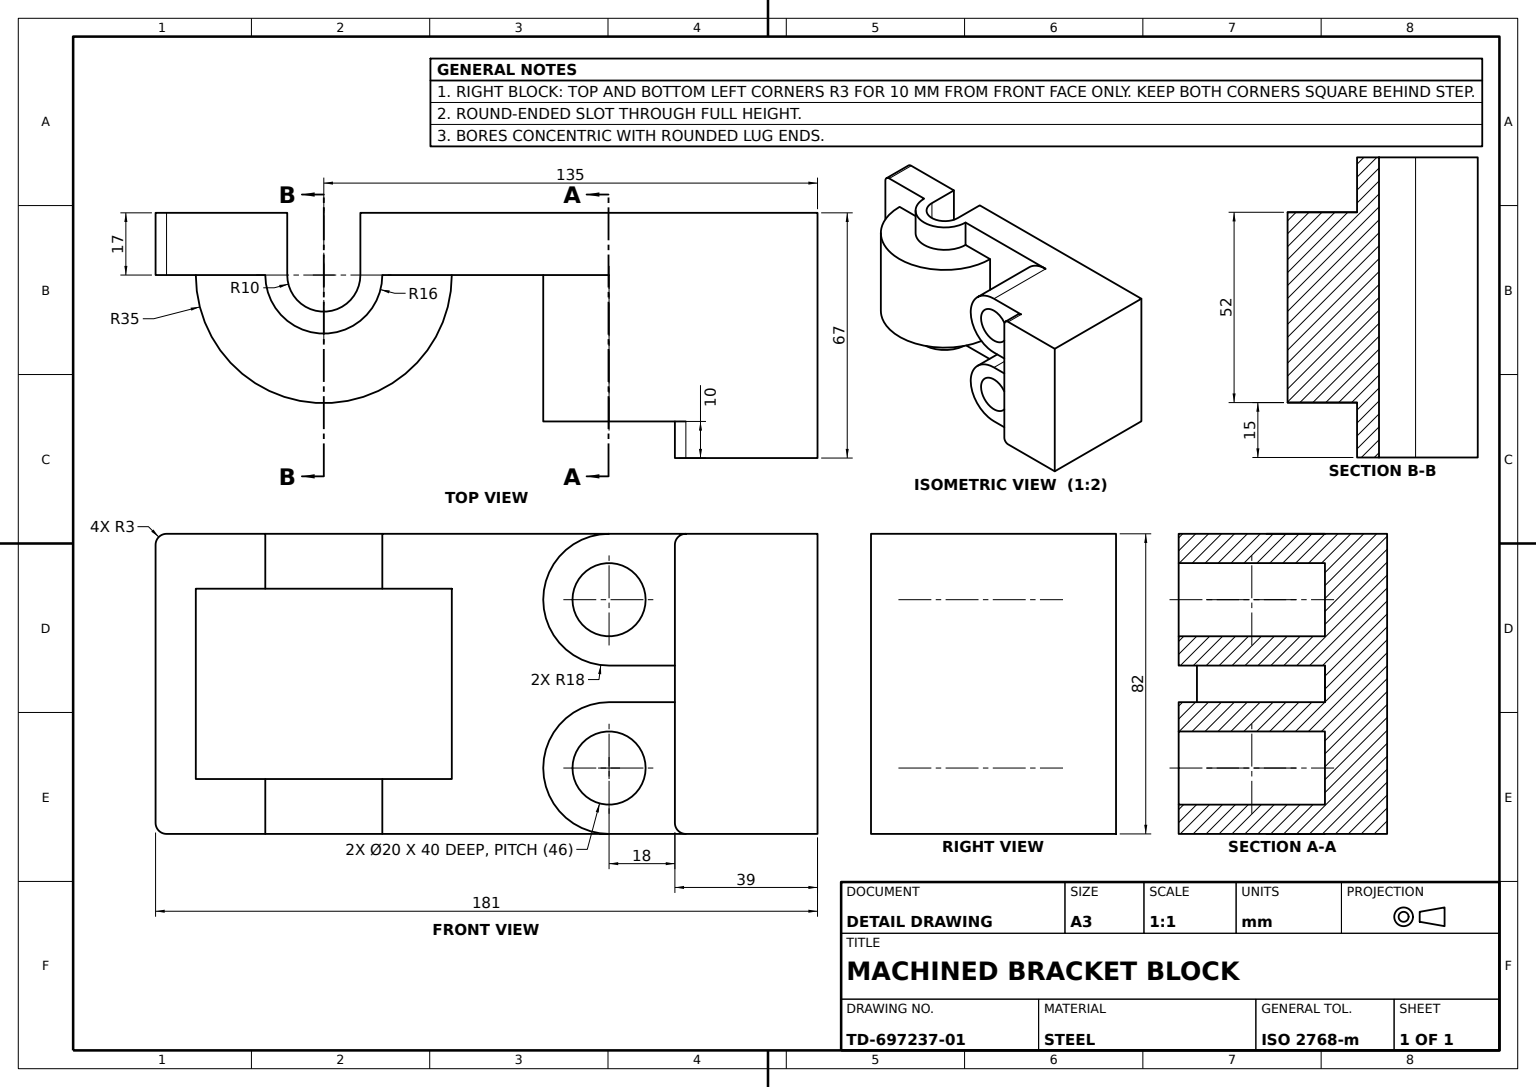
from build123d import *

# Parameters (mm, degrees)
BASE_BLOCK_SKETCH_W       = 175
BASE_BLOCK_SKETCH_H       = 82
BASE_BLOCK_DEPTH          = 17
SIDE_WALL_DEPTH           = 50
STEP_PAD_SKETCH_W         = 17
STEP_PAD_SKETCH_H         = 82
STEP_PAD_DEPTH            = 3
RAISED_BLOCK_DEPTH        = 17
LUG_BOSS_DEPTH            = 82
LUG_PROFILE_CUT_DEPTH     = 82
KNUCKLE_SLOT_1_DEPTH      = 15
KNUCKLE_START             = -15
KNUCKLE_SLOT_2_DEPTH      = 15
KNUCKLE_RING_2_DEPTH      = 15
KNUCKLE_START_2           = 15
KNUCKLE_RING_1_DEPTH      = 15
CURVED_BRACKET_DEPTH      = 40
BRACKET_TRIM_CUT_SKETCH_R = 10
BRACKET_TRIM_CUT_DEPTH    = 40


with BuildPart() as part:
    # Base Block Sketch → Base Block (new body)
    with BuildSketch(Plane.XY):
        with Locations((87.5, 41)):
            Rectangle(BASE_BLOCK_SKETCH_W, BASE_BLOCK_SKETCH_H)
    extrude(amount=BASE_BLOCK_DEPTH)

    # Side Wall Sketch → Side Wall (add)
    with BuildSketch(Plane.XY.offset(17)):
        with BuildLine():
            Line((175, 82), (175, 0))
            Line((175, 0), (139, 0))
            ThreePointArc((139, 0), (136.878679656, 0.878679656), (136, 3))
            Line((136, 3), (136, 79))
            ThreePointArc((136, 79), (136.878679656, 81.121320344), (139, 82))
            Line((139, 82), (175, 82))
        make_face()
    extrude(amount=SIDE_WALL_DEPTH)

    # Step Pad Sketch → Step Pad (add)
    with BuildSketch(Plane.ZY):
        with Locations((8.5, 41)):
            Rectangle(STEP_PAD_SKETCH_W, STEP_PAD_SKETCH_H)
    extrude(amount=STEP_PAD_DEPTH)

    # Raised Block Sketch → Raised Block (add)
    with BuildSketch(Plane.XY.offset(17)):
        with BuildLine():
            Line((-3, 82), (-3, 0))
            ThreePointArc((-3, 0), (-5.121320344, 0.878679656), (-6, 3))
            Line((-6, 3), (-6, 79))
            ThreePointArc((-6, 79), (-5.121320344, 81.121320344), (-3, 82))
        make_face()
    extrude(amount=-RAISED_BLOCK_DEPTH)

    # Lug Boss Sketch → Lug Boss (add)
    with BuildSketch(Plane.XZ):
        with BuildLine():
            ThreePointArc((75, 17), (40, 52), (5, 17))
            Line((5, 17), (75, 17))
        make_face()
    extrude(amount=-LUG_BOSS_DEPTH)

    # Lug Profile Cut Sketch → Lug Profile Cut (cut)
    with BuildSketch(Plane.XZ):
        with BuildLine():
            Line((30, 0), (50, 0))
            Line((50, 0), (50, 17))
            ThreePointArc((50, 17), (40, 27), (30, 17))
            Line((30, 17), (30, 0))
        make_face()
    extrude(amount=-LUG_PROFILE_CUT_DEPTH, mode=Mode.SUBTRACT)

    # Knuckle Slot 1 Sketch → Knuckle Slot 1 (cut)
    with BuildSketch(Plane.XZ):
        with BuildLine():
            Line((5, 17), (30, 17))
            ThreePointArc((30, 17), (40, 27), (50, 17))
            Line((50, 17), (75, 17))
            ThreePointArc((75, 17), (40, 52), (5, 17))
        make_face()
    extrude(amount=-KNUCKLE_SLOT_1_DEPTH, mode=Mode.SUBTRACT)

    # Knuckle Slot 2 Sketch → Knuckle Slot 2 (cut)
    with BuildSketch(Plane(origin=(0, 82, 0), x_dir=(1, 0, 0), z_dir=(0, 1, 0)).offset(KNUCKLE_START)):
        with BuildLine():
            Line((30, -17), (5, -17))
            ThreePointArc((5, -17), (40, -52), (75, -17))
            Line((75, -17), (50, -17))
            ThreePointArc((50, -17), (40, -27), (30, -17))
        make_face()
    extrude(amount=KNUCKLE_SLOT_2_DEPTH, mode=Mode.SUBTRACT)

    # Knuckle Ring 2 Sketch → Knuckle Ring 2 (add)
    with BuildSketch(Plane(origin=(0, 67, 0), x_dir=(1, 0, 0), z_dir=(0, 1, 0))):
        with BuildLine():
            Line((24, -17), (30, -17))
            ThreePointArc((30, -17), (40, -27), (50, -17))
            Line((50, -17), (56, -17))
            ThreePointArc((56, -17), (40, -33), (24, -17))
        make_face()
    extrude(amount=KNUCKLE_RING_2_DEPTH)

    # Knuckle Ring 1 Sketch → Knuckle Ring 1 (add)
    with BuildSketch(Plane.XZ.offset(-15).offset(KNUCKLE_START_2)):
        with BuildLine():
            Line((24, 17), (30, 17))
            ThreePointArc((30, 17), (40, 27), (50, 17))
            Line((50, 17), (56, 17))
            ThreePointArc((56, 17), (40, 33), (24, 17))
        make_face()
    extrude(amount=-KNUCKLE_RING_1_DEPTH)

    # Curved Bracket Sketch → Curved Bracket (add)
    with BuildSketch(Plane.XY.offset(17)):
        with BuildLine():
            Line((118, 0), (139, 0))
            ThreePointArc((139, 0), (136.878679656, 0.878679656), (136, 3))
            Line((136, 3), (136, 36))
            Line((136, 36), (118, 36))
            ThreePointArc((118, 36), (100, 18), (118, 0))
        make_face()
        with BuildLine():
            Line((118, 82), (139, 82))
            ThreePointArc((139, 82), (136.878679656, 81.121320344), (136, 79))
            Line((136, 79), (136, 46))
            Line((136, 46), (118, 46))
            ThreePointArc((118, 46), (100, 64), (118, 82))
        make_face()
    extrude(amount=CURVED_BRACKET_DEPTH)

    # Bracket Trim Cut Sketch → Bracket Trim Cut (cut)
    with BuildSketch(Plane.XY.offset(57)):
        with Locations((118, 64)):
            Circle(BRACKET_TRIM_CUT_SKETCH_R)
        with Locations((118, 18)):
            Circle(BRACKET_TRIM_CUT_SKETCH_R)
    extrude(amount=-BRACKET_TRIM_CUT_DEPTH, mode=Mode.SUBTRACT)


solid = part.part
